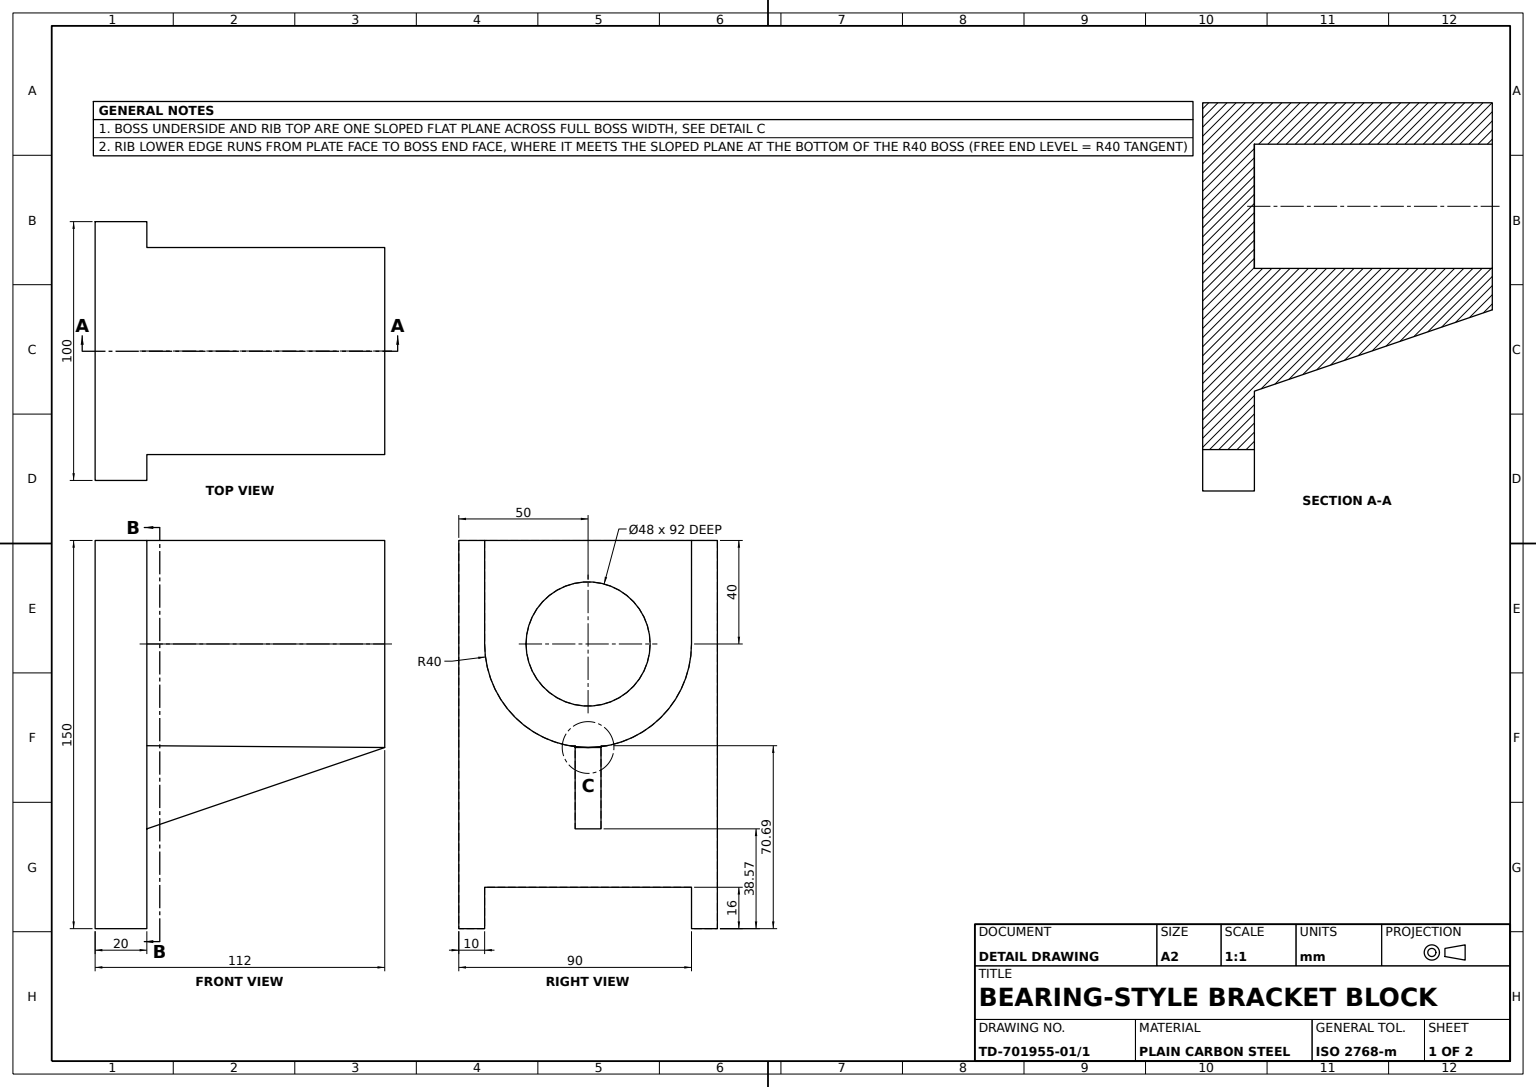
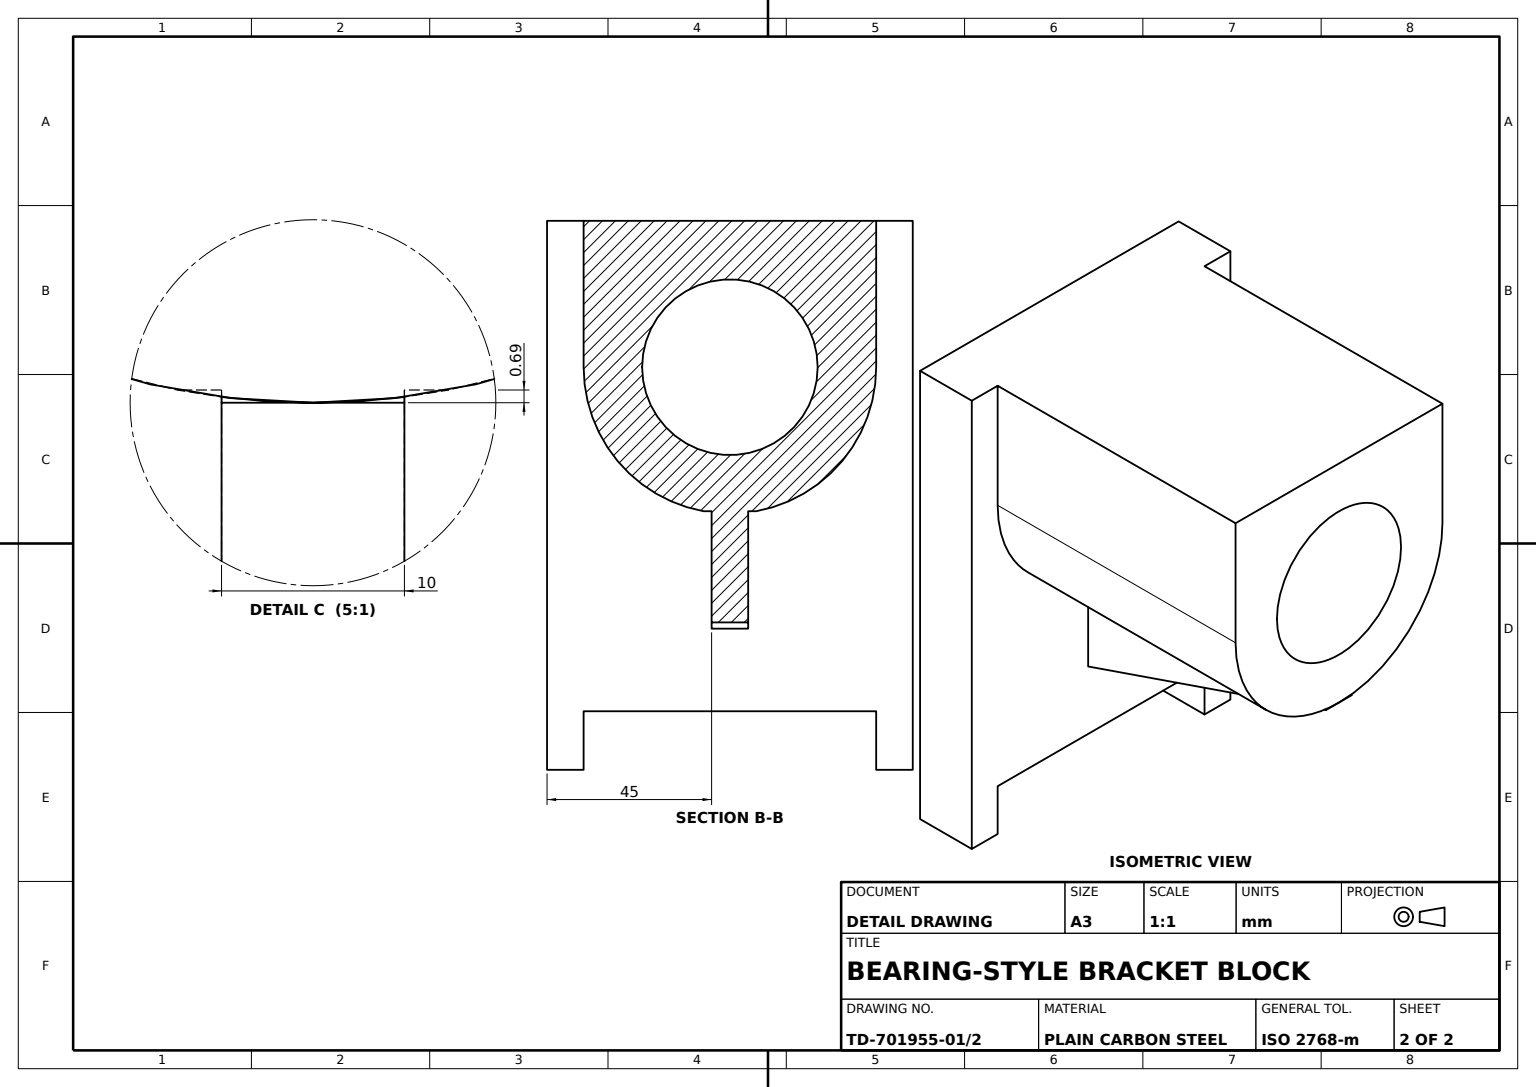
SolidWorks part; units mm, degrees
material "Plain Carbon Steel"
ref_plane "Front Plane" through (0, 0, 0) normal (0, 0, 1) x (1, 0, 0)
ref_plane "Top Plane" through (0, 0, 0) normal (0, 1, 0) x (1, 0, 0)
ref_plane "Right Plane" through (0, 0, 0) normal (1, 0, 0) x (0, 0, -1)
sketch "Base Plate Sketch" plane through (0, 0, 0) normal (0, 0, 1) x (1, 0, 0)
  line L0 (0, 0) -> (100, 0)
  line L1 (100, 0) -> (100, -150)
  line L2 (100, -150) -> (90, -150)
  line L3 (90, -150) -> (90, -134)
  line L4 (90, -134) -> (10, -134)
  line L5 (10, -134) -> (10, -150)
  line L6 (10, -150) -> (0, -150)
  line L7 (0, -150) -> (0, 0)
  dimension "D1" = 10
  dimension "D2" = 90
  dimension "D3" = 16
  dimension "D4" = 150
extrude "Base Plate 20mm" add sketch "Base Plate Sketch" along normal blind 20
sketch "Block Sketch" plane through (0, 0, 0) normal (0, 0, -1) x (-1, 0, 0)
  line L0 (0, 0) -> (0, -150) construction
  line L1 (-100, 0) -> (0, 0) construction
  line L2 (-10, -40) -> (-10, 0)
  line L3 (-10, 0) -> (-90, 0)
  line L4 (-90, 0) -> (-90, -40)
  arc A0 (-90, -40) -> (-10, -40) centre (-50, -40) ccw
  dimension "D1" = 80
  dimension "D2" = 40
  dimension "D3" = 50
extrude "Block 92mm" add sketch "Block Sketch" along normal blind 92
sketch "Relief Cut Sketch" plane through (0, 0, -92) normal (0, 0, -1) x (-1, 0, 0)
  circle A0 centre (-50, -40) radius 24
  dimension "D1" = 48
  dimension "D2" = 48
extrude "Relief Cut" cut sketch "Relief Cut Sketch" against normal blind 92
sketch "Gusset Sketch" plane through (0, 0, 0) normal (-1, 0, 0) x (0, 0, 1)
  line L0 (-92, -80) -> (0, -111.4294)
  line L1 (0, 0) -> (0, -150) construction
  line L2 (0, -111.4294) -> (0, -79.305)
  line L3 (0, -79.305) -> (-92, -80)
  line L4 (20, -150) -> (0, -150) construction
  dimension "D1" = 38.5706
  dimension "D2" = 70.695
extrude "Gusset 100mm" add sketch "Gusset Sketch" against normal blind 100
sketch "Gusset Trim Sketch 1" plane through (0, 0, 0) normal (-1, 0, 0) x (0, 0, 1)
  line L0 (-92, -80) -> (0, -79.305)
  line L1 (0, -79.305) -> (0, -111.4294)
  line L2 (0, -111.4294) -> (-92, -80)
extrude "Gusset Trim Cut 1" cut sketch "Gusset Trim Sketch 1" against normal blind 45
sketch "Gusset Trim Sketch 2" plane through (100, 0, 0) normal (1, 0, 0) x (0, 0, -1)
  line L0 (0, -79.305) -> (92, -80)
  line L1 (92, -80) -> (0, -111.4294)
  line L2 (0, -111.4294) -> (0, -79.305)
extrude "Gusset Trim Cut 2" cut sketch "Gusset Trim Sketch 2" against normal blind 45
